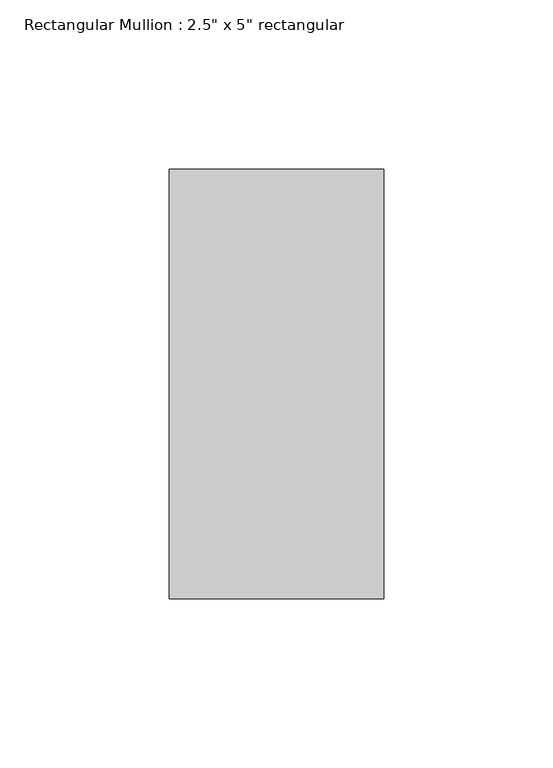
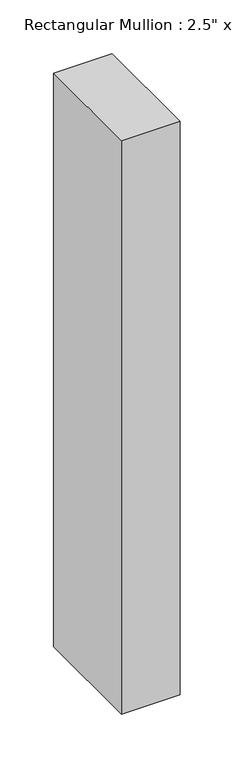
"""IFC4 building model written with IfcOpenShell, lengths in millimetres: member geometry."""

from ifc_helpers import new_model, si_unit, frame, origin, place, context, project, spatial, polyline, outline, extrude, source, transform, mapped, element, save


def member_7c181f63(model_context):
    return source(origin(), model_context, "Body", "SweptSolid", [
        extrude(outline(polyline([(0.0, 63.5), (0.0, -63.5), (-63.5, -63.5), (-63.5, 63.5), (0.0, 63.5)])), frame((0.0, 0.0, -654.05), z_axis=(0.0, 0.0, 1.0), x_axis=(1.0, 0.0, 0.0)), (0.0, 0.0, 1.0), 654.05),
    ])


if __name__ == "__main__":
    model = new_model("IFC4")
    model_context = context("Model", 3, world=origin())
    ifc_project = project(units=[si_unit("LENGTHUNIT", "METRE", prefix="MILLI")], contexts=[model_context])
    site = spatial("IfcSite", under=ifc_project)
    building = spatial("IfcBuilding", under=site)
    placement = place(None, origin())
    member_shape = member_7c181f63(model_context)
    element("IfcMember", 1, ObjectType="Rectangular Mullion : 2.5\" x 5\" rectangular", at=placement, inside=building, context=model_context, shape_type="MappedRepresentation", body=[
        mapped(member_shape, transform((0.0, 0.0, 0.0), x_axis=(1.0, 0.0, 0.0), y_axis=(0.0, 1.0, 0.0), z_axis=(0.0, 0.0, 1.0))),
    ])
    save(model, "model.ifc")

# Revit data of these elements
# Type "Rectangular Mullion : 2.5\" x 5\" rectangular"
#   built-in parameter 1007304 = 0.416667 (stored number, unit not read)
#   built-in parameter 1007301 = 0.104167 (stored number, unit not read)
#   built-in parameter 1007300 = 0.104167 (stored number, unit not read)
# Element 1 (IfcMember, "Rectangular Mullion : 2.5\" x 5\" rectangular")
#   Materials on its faces: "Aluminum"
# Materials
#   "Aluminum": class "Metal", colour RGB 247 247 247, transparency 0, Description = "Aluminum 6061", Cost = 0
